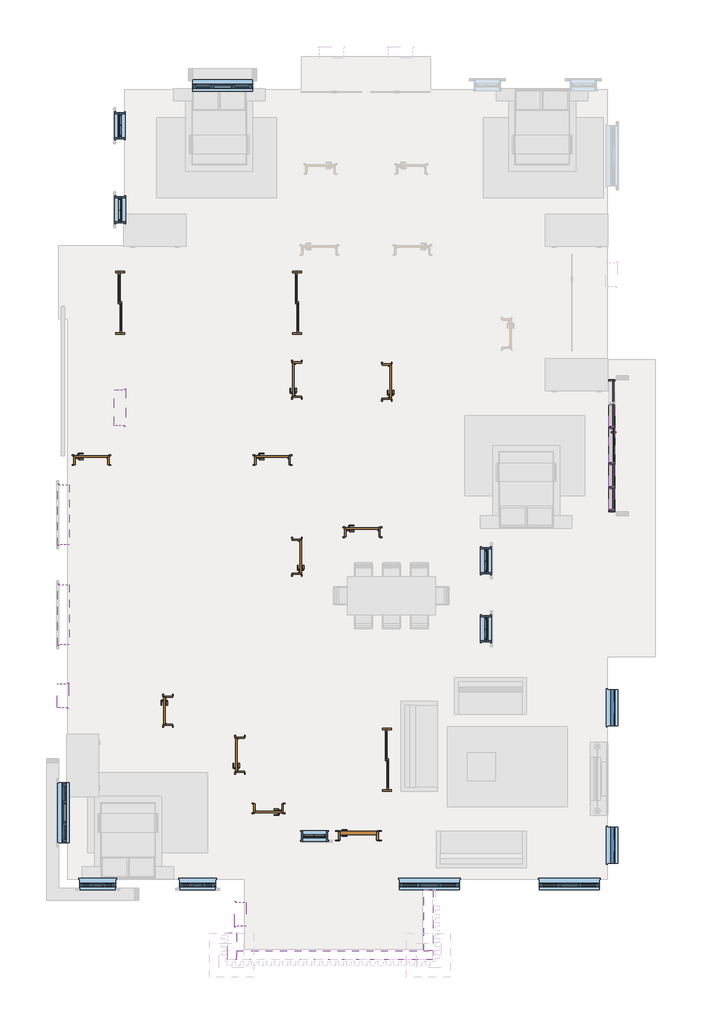
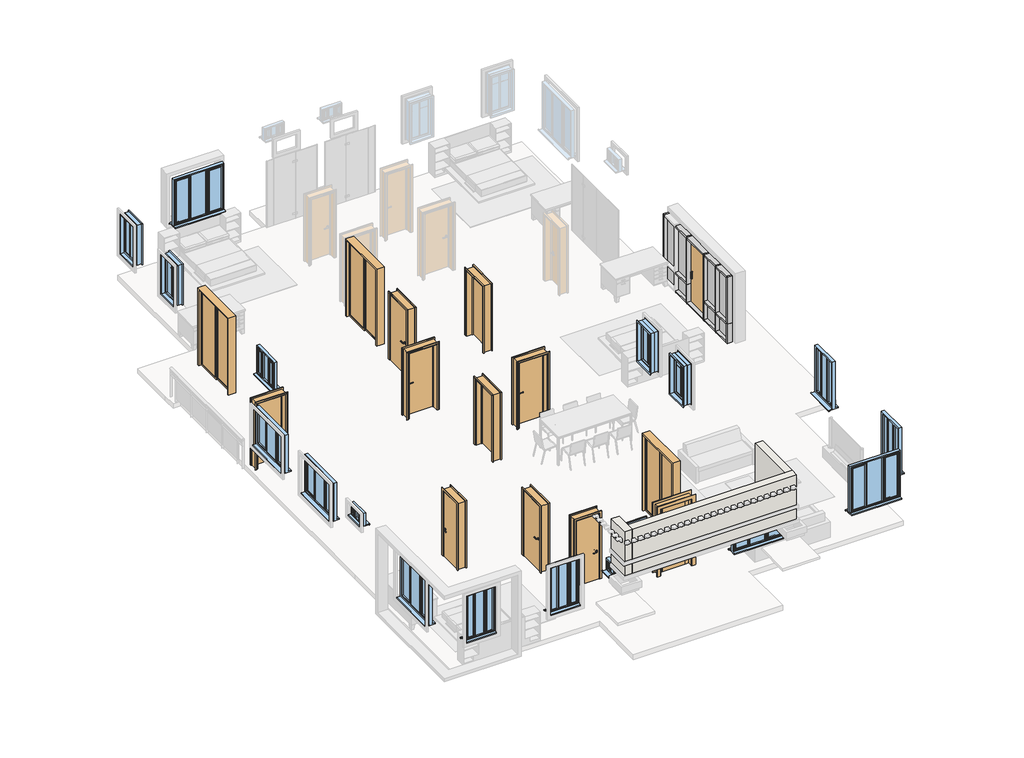
# One storey, part 1 of 2: 20 members, 18 windows, 14 doors, 8 plates, 3 walls.
"""IFC4 building model written with IfcOpenShell, lengths in millimetres."""

from ifc_helpers import new_model, si_unit, frame, origin, place, context, project, spatial, polyline, outline, extrude, faceted_brep, transform, mapped, element, save
from components import door_1500_x_2400mm_f3db478b, doors_intsgl_927b0b89, doors_intsgl_1caea894, doors_intsgl_900mm_doors_1c9cf9a6, doors_intsgl_900mm_doors_d21b38ee, m_door_curtain_wall_single_glass_m_door_curtain_wall_single_f8ee2cb8, single_flush_door_modern_12229_930_x_2100mm_fac4ccff, rectangular_mullion_50_x_150mm_5b5377e9, rectangular_mullion_50_x_150mm_de2b7ee4, rectangular_mullion_50_x_150mm_8a69f4a4, rectangular_mullion_50_x_150mm_b8dbbb25, rectangular_mullion_50_x_150mm_5dbd0429, rectangular_mullion_50_x_150mm_324a6438, rectangular_mullion_50_x_150mm_63369cdd, rectangular_mullion_50_x_150mm_7b69be1d, rectangular_mullion_50_x_150mm_c6835c94, system_panel_glazed_d134efab, system_panel_glazed_ea2acdbe, system_panel_glazed_163e0323, system_panel_glazed_68fefaed, tpl_plain_1500mm_wind_d4a9cd4c, tpl_plain_1500mm_wind_2_30e43110, tpl_plain_600mm_window_e9a44080, tpl_plain_900mm_wind_8db11632, tpl_plain_900mm_wind_2_fce8a64c, yu_window_casement_600x1200_84df8a12

model = new_model("IFC4")

# Units and contexts
model_context = context("Model", 3, world=origin())
ifc_project = project(units=[si_unit("LENGTHUNIT", "METRE", prefix="MILLI")], contexts=[model_context])

# Site, building, storey
site = spatial("IfcSite", under=ifc_project)
building = spatial("IfcBuilding", under=site)
storey = spatial("IfcBuildingStorey", under=building, Elevation=450.0)

# Doors
placement = place(None, origin())
door_1500_x_2400mm_shape = door_1500_x_2400mm_f3db478b(model_context)
element("IfcDoor", 1, ObjectType="1500 x 2400mm", at=placement, inside=storey, context=model_context, shape_type="MappedRepresentation", body=[
    mapped(door_1500_x_2400mm_shape, transform((-149.2953966, 3626.5650849, 450.0), x_axis=(0.0, -1.0, 0.0), y_axis=(1.0, 0.0, 0.0), z_axis=(0.0, 0.0, 1.0))),
])
element("IfcDoor", 2, ObjectType="1500 x 2400mm", at=placement, inside=storey, context=model_context, shape_type="MappedRepresentation", body=[
    mapped(door_1500_x_2400mm_shape, transform((-4574.2953966, 3626.5650849, 450.0), x_axis=(0.0, -1.0, 0.0), y_axis=(1.0, 0.0, 0.0), z_axis=(0.0, 0.0, 1.0))),
])
element("IfcDoor", 3, ObjectType="1500 x 2400mm", at=placement, inside=storey, context=model_context, shape_type="MappedRepresentation", body=[
    mapped(door_1500_x_2400mm_shape, transform((2100.7046034, -7795.9349151, 450.0), x_axis=(0.0, -1.0, 0.0), y_axis=(1.0, 0.0, 0.0), z_axis=(0.0, 0.0, 1.0))),
])
doors_intsgl_shape = doors_intsgl_927b0b89(model_context)
element("IfcDoor", 4, ObjectType="Doors_IntSgl", at=placement, inside=storey, context=model_context, shape_type="MappedRepresentation", body=[
    mapped(doors_intsgl_shape, transform((-3374.2953966, -6659.1929163, 450.0), x_axis=(0.0, -1.0, 0.0), y_axis=(1.0, 0.0, 0.0), z_axis=(0.0, 0.0, 1.0))),
])
doors_intsgl_2_shape = doors_intsgl_1caea894(model_context)
element("IfcDoor", 5, ObjectType="Doors_IntSgl", at=placement, inside=storey, context=model_context, shape_type="MappedRepresentation", body=[
    mapped(doors_intsgl_2_shape, transform((-861.7953966, -9096.6929163, 450.0), x_axis=(-1.0, 0.0, 0.0), y_axis=(0.0, -1.0, 0.0), z_axis=(0.0, 0.0, 1.0))),
])
doors_intsgl_900mm_doors_shape = doors_intsgl_900mm_doors_1c9cf9a6(model_context)
element("IfcDoor", 6, ObjectType="Doors_IntSgl : 900mm DOORS", at=placement, inside=storey, context=model_context, shape_type="MappedRepresentation", body=[
    mapped(doors_intsgl_900mm_doors_shape, transform((-5286.7953966, -396.6929163, 450.0), x_axis=(1.0, 0.0, 0.0), y_axis=(0.0, 1.0, 0.0), z_axis=(0.0, 0.0, 1.0))),
])
element("IfcDoor", 7, ObjectType="Doors_IntSgl : 900mm DOORS", at=placement, inside=storey, context=model_context, shape_type="MappedRepresentation", body=[
    mapped(doors_intsgl_900mm_doors_shape, transform((-761.7953966, -396.6929163, 450.0), x_axis=(1.0, 0.0, 0.0), y_axis=(0.0, 1.0, 0.0), z_axis=(0.0, 0.0, 1.0))),
])
element("IfcDoor", 8, ObjectType="Doors_IntSgl : 900mm DOORS", at=placement, inside=storey, context=model_context, shape_type="MappedRepresentation", body=[
    mapped(doors_intsgl_900mm_doors_shape, transform((1488.2046034, -2196.6929163, 450.0), x_axis=(1.0, 0.0, 0.0), y_axis=(0.0, 1.0, 0.0), z_axis=(0.0, 0.0, 1.0))),
])
element("IfcDoor", 9, ObjectType="Doors_IntSgl : 900mm DOORS", at=placement, inside=storey, context=model_context, shape_type="MappedRepresentation", body=[
    mapped(doors_intsgl_900mm_doors_shape, transform((-1574.2953966, -7759.1929163, 450.0), x_axis=(0.0, 1.0, 0.0), y_axis=(-1.0, 0.0, 0.0), z_axis=(0.0, 0.0, 1.0))),
])
element("IfcDoor", 10, ObjectType="Doors_IntSgl : 900mm DOORS", at=placement, inside=storey, context=model_context, shape_type="MappedRepresentation", body=[
    mapped(doors_intsgl_900mm_doors_shape, transform((-149.2953966, 1615.8070837, 450.0), x_axis=(0.0, 1.0, 0.0), y_axis=(-1.0, 0.0, 0.0), z_axis=(0.0, 0.0, 1.0))),
])
doors_intsgl_900mm_doors_2_shape = doors_intsgl_900mm_doors_d21b38ee(model_context)
element("IfcDoor", 11, ObjectType="Doors_IntSgl : 900mm DOORS", at=placement, inside=storey, context=model_context, shape_type="MappedRepresentation", body=[
    mapped(doors_intsgl_900mm_doors_2_shape, transform((-149.2953966, -2809.1929163, 450.0), x_axis=(0.0, 1.0, 0.0), y_axis=(-1.0, 0.0, 0.0), z_axis=(0.0, 0.0, 1.0))),
])
element("IfcDoor", 12, ObjectType="Doors_IntSgl : 900mm DOORS", at=placement, inside=storey, context=model_context, shape_type="MappedRepresentation", body=[
    mapped(doors_intsgl_900mm_doors_2_shape, transform((2100.7046034, 1565.8070837, 450.0), x_axis=(0.0, 1.0, 0.0), y_axis=(-1.0, 0.0, 0.0), z_axis=(0.0, 0.0, 1.0))),
])
m_door_curtain_wall_single_glass_m_door_curtain_wall_single_shape = m_door_curtain_wall_single_glass_m_door_curtain_wall_single_f8ee2cb8(model_context)
element("IfcDoor", 13, ObjectType="M_Door-Curtain-Wall-Single-Glass : M_Door-Curtain-Wall-Single-Glass", at=placement, inside=storey, context=model_context, shape_type="MappedRepresentation", body=[
    mapped(m_door_curtain_wall_single_glass_m_door_curtain_wall_single_shape, transform((7725.7046034, -34.1929163, 500.0), x_axis=(0.0, -1.0, 0.0), y_axis=(1.0, 0.0, 0.0), z_axis=(0.0, 0.0, 1.0))),
])
single_flush_door_modern_12229_930_x_2100mm_shape = single_flush_door_modern_12229_930_x_2100mm_fac4ccff(model_context)
element("IfcDoor", 14, ObjectType="Single_Flush_Door_-_Modern_12229 : 930 x 2100mm", at=placement, inside=storey, context=model_context, shape_type="MappedRepresentation", body=[
    mapped(single_flush_door_modern_12229_930_x_2100mm_shape, transform((1388.2046034, -9784.1929163, 450.0), x_axis=(-1.0, 0.0, 0.0), y_axis=(0.0, -1.0, 0.0), z_axis=(0.0, 0.0, 1.0))),
])

# Members
rectangular_mullion_50_x_150mm_shape = rectangular_mullion_50_x_150mm_5b5377e9(model_context)
element("IfcMember", 15, ObjectType="Rectangular Mullion : 50 x 150mm", at=placement, inside=storey, context=model_context, shape_type="MappedRepresentation", body=[
    mapped(rectangular_mullion_50_x_150mm_shape, transform((7725.7046034, -1634.1929163, 2550.0), x_axis=(0.0, 0.0, 1.0), y_axis=(-1.0, 0.0, 0.0), z_axis=(0.0, -1.0, 0.0))),
])
element("IfcMember", 16, ObjectType="Rectangular Mullion : 50 x 150mm", at=placement, inside=storey, context=model_context, shape_type="MappedRepresentation", body=[
    mapped(rectangular_mullion_50_x_150mm_shape, transform((7725.7046034, -1109.1929163, 450.0), x_axis=(0.0, 0.0, -1.0), y_axis=(-1.0, 0.0, 0.0), z_axis=(0.0, 1.0, 0.0))),
])
rectangular_mullion_50_x_150mm_2_shape = rectangular_mullion_50_x_150mm_de2b7ee4(model_context)
element("IfcMember", 17, ObjectType="Rectangular Mullion : 50 x 150mm", at=placement, inside=storey, context=model_context, shape_type="MappedRepresentation", body=[
    mapped(rectangular_mullion_50_x_150mm_2_shape, transform((7725.7046034, -1084.1929163, 450.0), x_axis=(0.0, -1.0, 0.0), y_axis=(-1.0, 0.0, 0.0), z_axis=(0.0, 0.0, -1.0))),
])
element("IfcMember", 18, ObjectType="Rectangular Mullion : 50 x 150mm", at=placement, inside=storey, context=model_context, shape_type="MappedRepresentation", body=[
    mapped(rectangular_mullion_50_x_150mm_2_shape, transform((7725.7046034, -484.1929163, 450.0), x_axis=(0.0, -1.0, 0.0), y_axis=(-1.0, 0.0, 0.0), z_axis=(0.0, 0.0, -1.0))),
])
element("IfcMember", 19, ObjectType="Rectangular Mullion : 50 x 150mm", at=placement, inside=storey, context=model_context, shape_type="MappedRepresentation", body=[
    mapped(rectangular_mullion_50_x_150mm_2_shape, transform((7725.7046034, 415.8070837, 450.0), x_axis=(0.0, -1.0, 0.0), y_axis=(-1.0, 0.0, 0.0), z_axis=(0.0, 0.0, -1.0))),
])
rectangular_mullion_50_x_150mm_3_shape = rectangular_mullion_50_x_150mm_8a69f4a4(model_context)
element("IfcMember", 20, ObjectType="Rectangular Mullion : 50 x 150mm", at=placement, inside=storey, context=model_context, shape_type="MappedRepresentation", body=[
    mapped(rectangular_mullion_50_x_150mm_3_shape, transform((7725.7046034, -1634.1929163, 1060.0), x_axis=(0.0, 0.0, 1.0), y_axis=(-1.0, 0.0, 0.0), z_axis=(0.0, -1.0, 0.0))),
])
rectangular_mullion_50_x_150mm_4_shape = rectangular_mullion_50_x_150mm_b8dbbb25(model_context)
element("IfcMember", 21, ObjectType="Rectangular Mullion : 50 x 150mm", at=placement, inside=storey, context=model_context, shape_type="MappedRepresentation", body=[
    mapped(rectangular_mullion_50_x_150mm_4_shape, transform((7725.7046034, -1059.1929163, 1060.0), x_axis=(0.0, 0.0, 1.0), y_axis=(-1.0, 0.0, 0.0), z_axis=(0.0, -1.0, 0.0))),
])
element("IfcMember", 22, ObjectType="Rectangular Mullion : 50 x 150mm", at=placement, inside=storey, context=model_context, shape_type="MappedRepresentation", body=[
    mapped(rectangular_mullion_50_x_150mm_4_shape, transform((7725.7046034, 440.8070837, 1060.0), x_axis=(0.0, 0.0, 1.0), y_axis=(-1.0, 0.0, 0.0), z_axis=(0.0, -1.0, 0.0))),
])
rectangular_mullion_50_x_150mm_5_shape = rectangular_mullion_50_x_150mm_5dbd0429(model_context)
element("IfcMember", 23, ObjectType="Rectangular Mullion : 50 x 150mm", at=placement, inside=storey, context=model_context, shape_type="MappedRepresentation", body=[
    mapped(rectangular_mullion_50_x_150mm_5_shape, transform((7725.7046034, -509.1929163, 450.0), x_axis=(0.0, 0.0, -1.0), y_axis=(-1.0, 0.0, 0.0), z_axis=(0.0, 1.0, 0.0))),
])
element("IfcMember", 24, ObjectType="Rectangular Mullion : 50 x 150mm", at=placement, inside=storey, context=model_context, shape_type="MappedRepresentation", body=[
    mapped(rectangular_mullion_50_x_150mm_5_shape, transform((7725.7046034, 990.8070837, 450.0), x_axis=(0.0, 0.0, -1.0), y_axis=(-1.0, 0.0, 0.0), z_axis=(0.0, 1.0, 0.0))),
])
rectangular_mullion_50_x_150mm_6_shape = rectangular_mullion_50_x_150mm_324a6438(model_context)
element("IfcMember", 25, ObjectType="Rectangular Mullion : 50 x 150mm", at=placement, inside=storey, context=model_context, shape_type="MappedRepresentation", body=[
    mapped(rectangular_mullion_50_x_150mm_6_shape, transform((7725.7046034, 390.8070837, 450.0), x_axis=(0.0, 0.0, -1.0), y_axis=(-1.0, 0.0, 0.0), z_axis=(0.0, 1.0, 0.0))),
])
element("IfcMember", 26, ObjectType="Rectangular Mullion : 50 x 150mm", at=placement, inside=storey, context=model_context, shape_type="MappedRepresentation", body=[
    mapped(rectangular_mullion_50_x_150mm_5_shape, transform((7725.7046034, -1059.1929163, 2550.0), x_axis=(0.0, 0.0, 1.0), y_axis=(-1.0, 0.0, 0.0), z_axis=(0.0, -1.0, 0.0))),
])
element("IfcMember", 27, ObjectType="Rectangular Mullion : 50 x 150mm", at=placement, inside=storey, context=model_context, shape_type="MappedRepresentation", body=[
    mapped(rectangular_mullion_50_x_150mm_5_shape, transform((7725.7046034, 440.8070837, 2550.0), x_axis=(0.0, 0.0, 1.0), y_axis=(-1.0, 0.0, 0.0), z_axis=(0.0, -1.0, 0.0))),
])
element("IfcMember", 28, ObjectType="Rectangular Mullion : 50 x 150mm", at=placement, inside=storey, context=model_context, shape_type="MappedRepresentation", body=[
    mapped(rectangular_mullion_50_x_150mm_6_shape, transform((7725.7046034, -459.1929163, 2550.0), x_axis=(0.0, 0.0, 1.0), y_axis=(-1.0, 0.0, 0.0), z_axis=(0.0, -1.0, 0.0))),
])
rectangular_mullion_50_x_150mm_7_shape = rectangular_mullion_50_x_150mm_63369cdd(model_context)
element("IfcMember", 29, ObjectType="Rectangular Mullion : 50 x 150mm", at=placement, inside=storey, context=model_context, shape_type="MappedRepresentation", body=[
    mapped(rectangular_mullion_50_x_150mm_7_shape, transform((7725.7046034, -1084.1929163, 1060.0), x_axis=(0.0, -1.0, 0.0), y_axis=(-1.0, 0.0, 0.0), z_axis=(0.0, 0.0, -1.0))),
])
element("IfcMember", 30, ObjectType="Rectangular Mullion : 50 x 150mm", at=placement, inside=storey, context=model_context, shape_type="MappedRepresentation", body=[
    mapped(rectangular_mullion_50_x_150mm_7_shape, transform((7725.7046034, -484.1929163, 1060.0), x_axis=(0.0, -1.0, 0.0), y_axis=(-1.0, 0.0, 0.0), z_axis=(0.0, 0.0, -1.0))),
])
element("IfcMember", 31, ObjectType="Rectangular Mullion : 50 x 150mm", at=placement, inside=storey, context=model_context, shape_type="MappedRepresentation", body=[
    mapped(rectangular_mullion_50_x_150mm_7_shape, transform((7725.7046034, 415.8070837, 1060.0), x_axis=(0.0, -1.0, 0.0), y_axis=(-1.0, 0.0, 0.0), z_axis=(0.0, 0.0, -1.0))),
])
rectangular_mullion_50_x_150mm_8_shape = rectangular_mullion_50_x_150mm_7b69be1d(model_context)
element("IfcMember", 32, ObjectType="Rectangular Mullion : 50 x 150mm", at=placement, inside=storey, context=model_context, shape_type="MappedRepresentation", body=[
    mapped(rectangular_mullion_50_x_150mm_8_shape, transform((7725.7046034, 1615.8070837, 2550.0), x_axis=(0.0, 1.0, 0.0), y_axis=(-1.0, 0.0, 0.0), z_axis=(0.0, 0.0, 1.0))),
])
rectangular_mullion_50_x_150mm_9_shape = rectangular_mullion_50_x_150mm_c6835c94(model_context)
element("IfcMember", 33, ObjectType="Rectangular Mullion : 50 x 150mm", at=placement, inside=storey, context=model_context, shape_type="MappedRepresentation", body=[
    mapped(rectangular_mullion_50_x_150mm_9_shape, transform((7725.7046034, -1684.1929163, 450.0), x_axis=(0.0, -1.0, 0.0), y_axis=(-1.0, 0.0, 0.0), z_axis=(0.0, 0.0, -1.0))),
])
element("IfcMember", 34, ObjectType="Rectangular Mullion : 50 x 150mm", at=placement, inside=storey, context=model_context, shape_type="MappedRepresentation", body=[
    mapped(rectangular_mullion_50_x_150mm_8_shape, transform((7725.7046034, -1684.1929163, 1060.0), x_axis=(0.0, -1.0, 0.0), y_axis=(-1.0, 0.0, 0.0), z_axis=(0.0, 0.0, -1.0))),
])

# Plates
system_panel_glazed_shape = system_panel_glazed_d134efab(model_context)
element("IfcPlate", 35, ObjectType="System Panel : Glazed", at=placement, inside=storey, context=model_context, shape_type="MappedRepresentation", body=[
    mapped(system_panel_glazed_shape, transform((7725.7046034, 1303.3070837, 500.0), x_axis=(0.0, -1.0, 0.0), y_axis=(1.0, 0.0, 0.0), z_axis=(0.0, 0.0, 1.0))),
])
element("IfcPlate", 36, ObjectType="System Panel : Glazed", at=placement, inside=storey, context=model_context, shape_type="MappedRepresentation", body=[
    mapped(system_panel_glazed_shape, transform((7725.7046034, -1371.6929163, 500.0), x_axis=(0.0, -1.0, 0.0), y_axis=(1.0, 0.0, 0.0), z_axis=(0.0, 0.0, 1.0))),
])
system_panel_glazed_2_shape = system_panel_glazed_ea2acdbe(model_context)
element("IfcPlate", 37, ObjectType="System Panel : Glazed", at=placement, inside=storey, context=model_context, shape_type="MappedRepresentation", body=[
    mapped(system_panel_glazed_2_shape, transform((7725.7046034, -784.1929163, 500.0), x_axis=(0.0, -1.0, 0.0), y_axis=(1.0, 0.0, 0.0), z_axis=(0.0, 0.0, 1.0))),
])
element("IfcPlate", 38, ObjectType="System Panel : Glazed", at=placement, inside=storey, context=model_context, shape_type="MappedRepresentation", body=[
    mapped(system_panel_glazed_2_shape, transform((7725.7046034, 715.8070837, 500.0), x_axis=(0.0, -1.0, 0.0), y_axis=(1.0, 0.0, 0.0), z_axis=(0.0, 0.0, 1.0))),
])
system_panel_glazed_3_shape = system_panel_glazed_163e0323(model_context)
element("IfcPlate", 39, ObjectType="System Panel : Glazed", at=placement, inside=storey, context=model_context, shape_type="MappedRepresentation", body=[
    mapped(system_panel_glazed_3_shape, transform((7725.7046034, 1303.3070837, 1085.0), x_axis=(0.0, -1.0, 0.0), y_axis=(1.0, 0.0, 0.0), z_axis=(0.0, 0.0, 1.0))),
])
element("IfcPlate", 40, ObjectType="System Panel : Glazed", at=placement, inside=storey, context=model_context, shape_type="MappedRepresentation", body=[
    mapped(system_panel_glazed_3_shape, transform((7725.7046034, -1371.6929163, 1085.0), x_axis=(0.0, -1.0, 0.0), y_axis=(1.0, 0.0, 0.0), z_axis=(0.0, 0.0, 1.0))),
])
system_panel_glazed_4_shape = system_panel_glazed_68fefaed(model_context)
element("IfcPlate", 41, ObjectType="System Panel : Glazed", at=placement, inside=storey, context=model_context, shape_type="MappedRepresentation", body=[
    mapped(system_panel_glazed_4_shape, transform((7725.7046034, 715.8070837, 1085.0), x_axis=(0.0, -1.0, 0.0), y_axis=(1.0, 0.0, 0.0), z_axis=(0.0, 0.0, 1.0))),
])
element("IfcPlate", 42, ObjectType="System Panel : Glazed", at=placement, inside=storey, context=model_context, shape_type="MappedRepresentation", body=[
    mapped(system_panel_glazed_4_shape, transform((7725.7046034, -784.1929163, 1085.0), x_axis=(0.0, -1.0, 0.0), y_axis=(1.0, 0.0, 0.0), z_axis=(0.0, 0.0, 1.0))),
])

# Walls
element("IfcWall", 43, ObjectType="225 wall", at=placement, inside=storey, context=model_context, shape_type="Brep", body=[
    faceted_brep([(-1879.2953966, -12209.1929163, 3150.0), (-1879.2953966, -12886.6929163, 3150.0), (-1879.2953966, -12886.6929163, 4650.0), (-1879.2953966, -12209.1929163, 4650.0), (-1654.2953966, -12209.1929163, 3150.0), (-1654.2953966, -12209.1929163, 4650.0), (-1654.2953966, -12661.6929163, 4650.0), (-1654.2953966, -12886.6929163, 4650.0), (-1654.2953966, -12886.6929163, 3150.0), (-1654.2953966, -12661.6929163, 3150.0)], [[[0, 1, 2, 3]], [[4, 5, 6, 7, 8, 9]], [[1, 0, 4, 9, 8]], [[3, 2, 7, 6, 5]], [[0, 3, 5, 4]], [[2, 1, 8, 7]]]),
])
element("IfcWall", 44, ObjectType="225 wall", at=placement, inside=storey, context=model_context, shape_type="Brep", body=[
    faceted_brep([(-1654.2953966, -12886.6929163, 3150.0), (3255.7046034, -12886.6929163, 3150.0), (3255.7046034, -12886.6929163, 4650.0), (-1654.2953966, -12886.6929163, 4650.0), (-1654.2953966, -12661.6929163, 3150.0), (-1654.2953966, -12661.6929163, 4650.0), (3030.7046034, -12661.6929163, 4650.0), (3255.7046034, -12661.6929163, 4650.0), (3255.7046034, -12661.6929163, 3150.0), (3030.7046034, -12661.6929163, 3150.0)], [[[0, 1, 2, 3]], [[4, 5, 6, 7, 8, 9]], [[1, 0, 4, 9, 8]], [[3, 2, 7, 6, 5]], [[0, 3, 5, 4]], [[2, 1, 8, 7]]]),
])
element("IfcWall", 45, ObjectType="225 wall", at=placement, inside=storey, context=model_context, shape_type="SweptSolid", body=[
    extrude(outline(polyline([(3030.7046034, -12661.6929163), (3030.7046034, -11134.1929163), (3255.7046034, -11134.1929163), (3255.7046034, -12661.6929163), (3030.7046034, -12661.6929163)])), frame((0.0, 0.0, 3150.0), z_axis=(0.0, 0.0, 1.0), x_axis=(1.0, 0.0, 0.0)), (0.0, 0.0, 1.0), 1500.0),
])

# Windows
tpl_plain_1500mm_wind_shape = tpl_plain_1500mm_wind_d4a9cd4c(model_context)
element("IfcWindow", 46, ObjectType="Tpl Plain : 1500mm wind", at=placement, inside=storey, context=model_context, shape_type="MappedRepresentation", body=[
    mapped(tpl_plain_1500mm_wind_shape, transform((-2536.7953966, 8986.7636515, 450.0), x_axis=(-1.0, 0.0, 0.0), y_axis=(0.0, -1.0, 0.0), z_axis=(0.0, 0.0, 1.0))),
])
element("IfcWindow", 47, ObjectType="Tpl Plain : 1500mm wind", at=placement, inside=storey, context=model_context, shape_type="MappedRepresentation", body=[
    mapped(tpl_plain_1500mm_wind_shape, transform((-6007.7519645, -9734.1929163, 450.0), x_axis=(0.0, -1.0, 0.0), y_axis=(1.0, 0.0, 0.0), z_axis=(0.0, 0.0, 1.0))),
])
element("IfcWindow", 48, ObjectType="Tpl Plain : 1500mm wind", at=placement, inside=storey, context=model_context, shape_type="MappedRepresentation", body=[
    mapped(tpl_plain_1500mm_wind_shape, transform((2638.2046034, -10975.7363485, 450.0), x_axis=(-1.0, 0.0, 0.0), y_axis=(0.0, -1.0, 0.0), z_axis=(0.0, 0.0, 1.0))),
])
element("IfcWindow", 49, ObjectType="Tpl Plain : 1500mm wind", at=placement, inside=storey, context=model_context, shape_type="MappedRepresentation", body=[
    mapped(tpl_plain_1500mm_wind_shape, transform((6138.2046034, -10975.7363485, 450.0), x_axis=(-1.0, 0.0, 0.0), y_axis=(0.0, -1.0, 0.0), z_axis=(0.0, 0.0, 1.0))),
])
tpl_plain_1500mm_wind_2_shape = tpl_plain_1500mm_wind_2_30e43110(model_context)
element("IfcWindow", 50, ObjectType="Tpl Plain : 1500mm wind 2", at=placement, inside=storey, context=model_context, shape_type="MappedRepresentation", body=[
    mapped(tpl_plain_1500mm_wind_2_shape, transform((-6007.7519645, -2284.1929163, 450.0), x_axis=(0.0, -1.0, 0.0), y_axis=(1.0, 0.0, 0.0), z_axis=(0.0, 0.0, 1.0))),
])
element("IfcWindow", 51, ObjectType="Tpl Plain : 1500mm wind 2", at=placement, inside=storey, context=model_context, shape_type="MappedRepresentation", body=[
    mapped(tpl_plain_1500mm_wind_2_shape, transform((-6007.7519645, -4784.1929163, 450.0), x_axis=(0.0, -1.0, 0.0), y_axis=(1.0, 0.0, 0.0), z_axis=(0.0, 0.0, 1.0))),
])
tpl_plain_600mm_window_shape = tpl_plain_600mm_window_e9a44080(model_context)
element("IfcWindow", 52, ObjectType="Tpl Plain : 600mm window", at=placement, inside=storey, context=model_context, shape_type="MappedRepresentation", body=[
    mapped(tpl_plain_600mm_window_shape, transform((-1582.7519645, -12119.1929163, 450.0), x_axis=(0.0, -1.0, 0.0), y_axis=(1.0, 0.0, 0.0), z_axis=(0.0, 0.0, 1.0))),
])
element("IfcWindow", 53, ObjectType="Tpl Plain : 600mm window", at=placement, inside=storey, context=model_context, shape_type="MappedRepresentation", body=[
    mapped(tpl_plain_600mm_window_shape, transform((-5990.8388288, -5909.1929163, 450.0), x_axis=(0.0, 1.0, 0.0), y_axis=(-1.0, 0.0, 0.0), z_axis=(0.0, 0.0, 1.0))),
])
tpl_plain_900mm_wind_shape = tpl_plain_900mm_wind_8db11632(model_context)
element("IfcWindow", 54, ObjectType="Tpl Plain : 900mm wind", at=placement, inside=storey, context=model_context, shape_type="MappedRepresentation", body=[
    mapped(tpl_plain_900mm_wind_shape, transform((-4565.8388288, 1340.8070837, 450.0), x_axis=(0.0, 1.0, 0.0), y_axis=(-1.0, 0.0, 0.0), z_axis=(0.0, 0.0, 1.0))),
])
tpl_plain_900mm_wind_2_shape = tpl_plain_900mm_wind_2_fce8a64c(model_context)
element("IfcWindow", 55, ObjectType="Tpl Plain : 900mm wind 2", at=placement, inside=storey, context=model_context, shape_type="MappedRepresentation", body=[
    mapped(tpl_plain_900mm_wind_2_shape, transform((7717.2480355, -10446.6929163, 690.0), x_axis=(0.0, -1.0, 0.0), y_axis=(1.0, 0.0, 0.0), z_axis=(0.0, 0.0, 1.0))),
])
element("IfcWindow", 56, ObjectType="Tpl Plain : 900mm wind 2", at=placement, inside=storey, context=model_context, shape_type="MappedRepresentation", body=[
    mapped(tpl_plain_900mm_wind_2_shape, transform((7717.2480355, -7009.1929163, 690.0), x_axis=(0.0, -1.0, 0.0), y_axis=(1.0, 0.0, 0.0), z_axis=(0.0, 0.0, 1.0))),
])
element("IfcWindow", 57, ObjectType="Tpl Plain : 900mm wind 2", at=placement, inside=storey, context=model_context, shape_type="MappedRepresentation", body=[
    mapped(tpl_plain_900mm_wind_2_shape, transform((-3061.7953966, -10975.7363485, 450.0), x_axis=(-1.0, 0.0, 0.0), y_axis=(0.0, -1.0, 0.0), z_axis=(0.0, 0.0, 1.0))),
])
element("IfcWindow", 58, ObjectType="Tpl Plain : 900mm wind 2", at=placement, inside=storey, context=model_context, shape_type="MappedRepresentation", body=[
    mapped(tpl_plain_900mm_wind_2_shape, transform((-5561.7953966, -10975.7363485, 450.0), x_axis=(-1.0, 0.0, 0.0), y_axis=(0.0, -1.0, 0.0), z_axis=(0.0, 0.0, 1.0))),
])
yu_window_casement_600x1200_shape = yu_window_casement_600x1200_84df8a12(model_context)
element("IfcWindow", 59, ObjectType="Yu_Window : Casement 600x1200", at=placement, inside=storey, context=model_context, shape_type="MappedRepresentation", body=[
    mapped(yu_window_casement_600x1200_shape, transform((-4574.2953966, 7965.8070837, 990.0), x_axis=(0.0, 1.0, 0.0), y_axis=(-1.0, 0.0, 0.0), z_axis=(0.0, 0.0, 1.0))),
])
element("IfcWindow", 60, ObjectType="Yu_Window : Casement 600x1200", at=placement, inside=storey, context=model_context, shape_type="MappedRepresentation", body=[
    mapped(yu_window_casement_600x1200_shape, transform((-4574.2953966, 5865.8070837, 990.0), x_axis=(0.0, -1.0, 0.0), y_axis=(1.0, 0.0, 0.0), z_axis=(0.0, 0.0, 1.0))),
])
element("IfcWindow", 61, ObjectType="Yu_Window : Casement 600x1200", at=placement, inside=storey, context=model_context, shape_type="MappedRepresentation", body=[
    mapped(yu_window_casement_600x1200_shape, transform((4575.7046034, -2909.1929163, 990.0), x_axis=(0.0, -1.0, 0.0), y_axis=(1.0, 0.0, 0.0), z_axis=(0.0, 0.0, 1.0))),
])
element("IfcWindow", 62, ObjectType="Yu_Window : Casement 600x1200", at=placement, inside=storey, context=model_context, shape_type="MappedRepresentation", body=[
    mapped(yu_window_casement_600x1200_shape, transform((4575.7046034, -4609.1929163, 990.0), x_axis=(0.0, -1.0, 0.0), y_axis=(1.0, 0.0, 0.0), z_axis=(0.0, 0.0, 1.0))),
])
element("IfcWindow", 63, ObjectType="Yu_Window : Casement 600x1200", at=placement, inside=storey, context=model_context, shape_type="MappedRepresentation", body=[
    mapped(yu_window_casement_600x1200_shape, transform((288.2046034, -9784.1929163, 450.0), x_axis=(-1.0, 0.0, 0.0), y_axis=(0.0, -1.0, 0.0), z_axis=(0.0, 0.0, 1.0))),
])

save(model, "model.ifc")

# Revit data of these elements
# Type "1500 x 2400mm"
#   Type Mark = "47"
#   Operation = "UserDefined"
#   Analytic Construction = "<None>"
#   Width = 1500 mm
#   Thickness = 40 mm
#   Rough Width = 1580 mm
#   Rough Height = 2440 mm
#   Panel Width = 777.5 mm
#   Panel Frame = 55 mm
#   Height = 2400 mm
#   Frame Depth = 40 mm
#   Define Thermal Properties by = 1
#   Glass Material = Sliding Door Glass
#   Frame Material = Sliding Door Frame
#   Function = (empty or 0)
# Type "Doors_IntSgl"
#   Type Mark = "45"
#   Type Comments = "Internal Single"
#   Operation = "SingleSwingRight"
#   Manufacturer = "Revit"
#   Keynote = "L20"
#   Description = "Internal Single Door"
#   Analytic Construction = "Metal"
#   UnderCut = 8 mm
#   Tolerance = 2 mm
#   Thickness = 38 mm
#   Thermal Resistance (R) = 0.270117 (m²·K)/W
#   Structural Tolerance = 8 mm
#   StopDepth = 32 mm
#   Stop Thickness = 19 mm
#   Rough Width = 750 mm
#   Rough Height = 2100 mm
#   Height to Top Lock Rail = 1000 mm
#   Heat Transfer Coefficient (U) = 3.7021 W/(m²·K)
#   Handle Z Distance = 900 mm
#   Handle X Distance = 75 mm
#   Frame Thickness = 32 mm
#   Door Panel Width = 666 mm
#   Door Panel Thickness = 38 mm
#   Door Panel Offset = 0 mm
#   Height = 2100 mm
#   Width = 750 mm
#   Door Panel Height = 2050 mm
#   Architrave Setback = 5 mm
#   Vis - Ironmongery = yes
#   Define Thermal Properties by = 1
#   Material Ironmongery = Door - Handle
#   Material Frame = Door - Frame/Mullion (1)
#   Material Door = Door - Panel
#   Material Architrave = Door - Architrave
#   Visual Light Transmittance = 0
#   Solar Heat Gain Coefficient = 0
#   Function = (empty or 0)
#   Wall Closure = (empty or 0)
# Type "Doors_IntSgl : 900mm DOORS"
#   Type Mark = "46"
#   Type Comments = "Internal Single"
#   Operation = "SingleSwingRight"
#   Manufacturer = "Revit"
#   Keynote = "L20"
#   Description = "Internal Single Door"
#   Analytic Construction = "Metal"
#   UnderCut = 8 mm
#   Tolerance = 2 mm
#   Thickness = 38 mm
#   Thermal Resistance (R) = 0.270117 (m²·K)/W
#   Structural Tolerance = 8 mm
#   StopDepth = 32 mm
#   Stop Thickness = 19 mm
#   Rough Width = 900 mm
#   Rough Height = 2100 mm
#   Height to Top Lock Rail = 1000 mm
#   Heat Transfer Coefficient (U) = 3.7021 W/(m²·K)
#   Handle Z Distance = 1000 mm
#   Handle X Distance = 75 mm
#   Frame Thickness = 32 mm
#   Door Panel Width = 816 mm
#   Door Panel Thickness = 38 mm
#   Door Panel Offset = 0 mm
#   Height = 2100 mm
#   Width = 900 mm
#   Door Panel Height = 2050 mm
#   Architrave Setback = 5 mm
#   Vis - Ironmongery = yes
#   Define Thermal Properties by = 1
#   Material Ironmongery = Door - Handle
#   Material Frame = Door - Frame/Mullion (1)
#   Material Door = Door - Panel
#   Material Architrave = Door - Architrave
#   Visual Light Transmittance = 0
#   Solar Heat Gain Coefficient = 0
#   Function = (empty or 0)
#   Wall Closure = (empty or 0)
# Type "M_Door-Curtain-Wall-Single-Glass : M_Door-Curtain-Wall-Single-Glass"
#   Type Mark = "51"
#   Assembly Code = "B2030100"
#   Analytic Construction = "<None>"
#   Width [instance default] = 900 mm
#   Thermal Resistance (R) = 1.7611 (m²·K)/W
#   Swing Angle [instance default] = 90.00°
#   Heat Transfer Coefficient (U) = 0.567826 W/(m²·K)
#   Offset = 50.8 mm
#   Define Thermal Properties by = 1
#   Function = 1
#   Door Handle Material = Aluminum
#   Glazing = Glass
#   Visual Light Transmittance = 0
#   Solar Heat Gain Coefficient = 0
#   Construction Type Id = ""
# Type "Single_Flush_Door_-_Modern_12229 : 930 x 2100mm"
#   Type Mark = "50"
#   Description = "HWD FRAMED & PANELLED SINGLE DOOR"
#   Analytic Construction = "<None>"
#   Thickness = 45 mm
#   Rough Width = 1000 mm
#   Rough Height = 2145 mm
#   Frame Projection Ext. = 10 mm
#   Frame Projection Int. = 10 mm
#   Frame Width = 75 mm
#   Height = 2100 mm
#   Width = 930 mm
#   Define Thermal Properties by = 1
#   Jamb Material = Window Frame
#   Door Material = Window Frame
#   Function = (empty or 0)
#   Wall Closure = (empty or 0)
#   Assembly Code = ""
# Type "Rectangular Mullion : 50 x 150mm"
#   built-in parameter 1007304 = 0.492126 (stored number, unit not read)
#   built-in parameter 1007301 = 0.082021 (stored number, unit not read)
#   built-in parameter 1007300 = 0.082021 (stored number, unit not read)
# Type "System Panel : Glazed"
#   Construction Type Id = "GSP4R"
#   Analytic Construction = "1/8 in Pilkington single glazing"
#   Visual Light Transmittance = 0.9
#   Solar Heat Gain Coefficient = 0.86
#   Heat Transfer Coefficient (U) = 6.7069 W/(m²·K)
#   Define Thermal Properties by = 1
# Type "225 wall"
#   Layers, outside or top first: 225 mm "Concrete, Cast In Situ" (function 1)
# Type "Tpl Plain : 1500mm wind"
#   Type Mark = "34"
#   Operation = "TriplePanelVertical"
#   Manufacturer = "Revit"
#   Keynote = "L10"
#   Analytic Construction = "<None>"
#   Wrap Layers (Ext) from Ext = 102.5 mm
#   Wrap Layers (Int) from Ext = 177.5 mm
#   Window Board Projection = 25 mm
#   Window Board Extension = 25 mm
#   Rough Width = 1500 mm
#   Rough Height = 1500 mm
#   Height = 1500 mm
#   Width = 1500 mm
#   Glazing Thickness = 24 mm
#   FrameOffset - External = 50 mm
#   Frame Depth = 65 mm
#   Default Head Height = 2400 mm
#   Cill Depth = 87.5 mm
#   Cavity Closer Width = 50 mm
#   Cavity Closer Offset from Ext = 102.5 mm
#   Cavity Closer Depth = 85 mm
#   Vis - Cavity Closers = yes
#   Define Thermal Properties by = 1
#   Material Trim = Window Frame
#   Material Glass = Glass
#   Material Frame = Window Frame
#   Wall Closure = (empty or 0)
# Type "Tpl Plain : 1500mm wind 2"
#   Type Mark = "37"
#   Operation = "TriplePanelVertical"
#   Manufacturer = "Revit"
#   Keynote = "L10"
#   Analytic Construction = "<None>"
#   Wrap Layers (Ext) from Ext = 102.5 mm
#   Wrap Layers (Int) from Ext = 177.5 mm
#   Window Board Projection = 25 mm
#   Window Board Extension = 25 mm
#   Rough Width = 1500 mm
#   Rough Height = 1200 mm
#   Height = 1200 mm
#   Width = 1500 mm
#   Glazing Thickness = 24 mm
#   FrameOffset - External = 50 mm
#   Frame Depth = 65 mm
#   Default Head Height = 2400 mm
#   Cill Depth = 87.5 mm
#   Cavity Closer Width = 50 mm
#   Cavity Closer Offset from Ext = 102.5 mm
#   Cavity Closer Depth = 85 mm
#   Vis - Cavity Closers = yes
#   Define Thermal Properties by = 1
#   Material Trim = Window Frame
#   Material Glass = Glass
#   Material Frame = Window Frame
#   Wall Closure = (empty or 0)
# Type "Tpl Plain : 600mm window"
#   Type Mark = "33"
#   Operation = "TriplePanelVertical"
#   Manufacturer = "Revit"
#   Keynote = "L10"
#   Analytic Construction = "<None>"
#   Wrap Layers (Ext) from Ext = 102.5 mm
#   Wrap Layers (Int) from Ext = 177.5 mm
#   Window Board Projection = 25 mm
#   Window Board Extension = 25 mm
#   Rough Width = 600 mm
#   Rough Height = 400 mm
#   Height = 400 mm
#   Width = 600 mm
#   Glazing Thickness = 24 mm
#   FrameOffset - External = 50 mm
#   Frame Depth = 65 mm
#   Default Head Height = 2400 mm
#   Cill Depth = 87.5 mm
#   Cavity Closer Width = 50 mm
#   Cavity Closer Offset from Ext = 102.5 mm
#   Cavity Closer Depth = 85 mm
#   Vis - Cavity Closers = yes
#   Define Thermal Properties by = 1
#   Material Trim = Window Frame
#   Material Glass = Glass
#   Material Frame = Window Frame
#   Wall Closure = (empty or 0)
# Type "Tpl Plain : 900mm wind"
#   Type Mark = "35"
#   Operation = "TriplePanelVertical"
#   Manufacturer = "Revit"
#   Keynote = "L10"
#   Analytic Construction = "<None>"
#   Wrap Layers (Ext) from Ext = 102.5 mm
#   Wrap Layers (Int) from Ext = 177.5 mm
#   Window Board Projection = 25 mm
#   Window Board Extension = 25 mm
#   Rough Width = 900 mm
#   Rough Height = 900 mm
#   Height = 900 mm
#   Width = 900 mm
#   Glazing Thickness = 24 mm
#   FrameOffset - External = 50 mm
#   Frame Depth = 65 mm
#   Default Head Height = 2400 mm
#   Cill Depth = 87.5 mm
#   Cavity Closer Width = 50 mm
#   Cavity Closer Offset from Ext = 102.5 mm
#   Cavity Closer Depth = 85 mm
#   Vis - Cavity Closers = yes
#   Define Thermal Properties by = 1
#   Material Trim = Window Frame
#   Material Glass = Glass
#   Material Frame = Window Frame
#   Wall Closure = (empty or 0)
# Type "Tpl Plain : 900mm wind 2"
#   Type Mark = "36"
#   Operation = "TriplePanelVertical"
#   Manufacturer = "Revit"
#   Keynote = "L10"
#   Analytic Construction = "<None>"
#   Wrap Layers (Ext) from Ext = 102.5 mm
#   Wrap Layers (Int) from Ext = 177.5 mm
#   Window Board Projection = 25 mm
#   Window Board Extension = 25 mm
#   Rough Width = 900 mm
#   Rough Height = 1500 mm
#   Height = 1500 mm
#   Width = 900 mm
#   Glazing Thickness = 24 mm
#   FrameOffset - External = 50 mm
#   Frame Depth = 65 mm
#   Default Head Height = 2400 mm
#   Cill Depth = 87.5 mm
#   Cavity Closer Width = 50 mm
#   Cavity Closer Offset from Ext = 102.5 mm
#   Cavity Closer Depth = 85 mm
#   Vis - Cavity Closers = yes
#   Define Thermal Properties by = 1
#   Material Trim = Window Frame
#   Material Glass = Glass
#   Material Frame = Window Frame
#   Wall Closure = (empty or 0)
# Type "Yu_Window : Casement 600x1200"
#   Type Mark = "28"
#   Analytic Construction = "<None>"
#   mullion 2 = 300 mm
#   Window panel size 1 = 300 mm
#   Offset = 25 mm
#   Height = 1200 mm
#   Default Sill Height = 600 mm
#   Width = 600 mm
#   Define Thermal Properties by = 1
#   Interior material = none
#   Exterior material = none
#   Wall Closure = (empty or 0)
# Elements 1, 2, 3 (IfcDoor, "1500 x 2400mm")
#   Phase Created = New Construction
#   Materials on its faces: "Sliding Door Frame", "Sliding Door Glass"
# Elements 4, 5 (IfcDoor, "Doors_IntSgl")
#   Phase Created = New Construction
#   Materials on its faces: "Door - Architrave", "Door - Handle", "Door - Frame/Mullion (1)", "Door - Panel"
# Elements 6, 7, 8, 9, 10, 11, 12 (IfcDoor, "Doors_IntSgl : 900mm DOORS")
#   Phase Created = New Construction
#   Materials on its faces: "Door - Architrave", "Door - Handle", "Door - Frame/Mullion (1)", "Door - Panel"
# Element 13 (IfcDoor, "M_Door-Curtain-Wall-Single-Glass : M_Door-Curtain-Wall-Single-Glass")
#   Phase Created = New Construction
#   Materials on its faces: "Aluminum", "Glass"
# Element 14 (IfcDoor, "Single_Flush_Door_-_Modern_12229 : 930 x 2100mm")
#   Phase Created = New Construction
#   Materials on its faces: "Window Frame"
# Elements 15, 16, 17, 18, 19, 20, 21, 22, 23, 24, 25, 26, 27, 28, 29, 30, 31, 32, 33, 34 (IfcMember, "Rectangular Mullion : 50 x 150mm")
#   Phase Created = New Construction
#   Materials on its faces: "Aluminium"
# Elements 35, 36, 37, 38, 39, 40, 41, 42 (IfcPlate, "System Panel : Glazed")
#   Phase Created = New Construction
#   Materials on its faces: "Glass"
# Elements 43, 44, 45 (IfcWall, "225 wall")
#   built-in parameter 1001111 = 2700 mm
#   Top Offset = 600 mm
#   Base Offset = 2700 mm
#   wall height = 1500 mm
#   Phase Created = New Construction
#   Base Constraint = 01-DPC
#   Top Constraint = 3-ROOF
#   Materials on its faces: "Concrete, Cast In Situ"
# Element 46 (IfcWindow, "Tpl Plain : 1500mm wind")
#   Mark = "6"
#   Phase Created = New Construction
#   Materials on its faces: "Window Frame", "Glass"
# Element 47 (IfcWindow, "Tpl Plain : 1500mm wind")
#   Mark = "9"
#   Phase Created = New Construction
#   Materials on its faces: "Window Frame", "Glass"
# Element 48 (IfcWindow, "Tpl Plain : 1500mm wind")
#   Mark = "18"
#   Phase Created = New Construction
#   Materials on its faces: "Window Frame", "Glass"
# Element 49 (IfcWindow, "Tpl Plain : 1500mm wind")
#   Mark = "19"
#   Phase Created = New Construction
#   Materials on its faces: "Window Frame", "Glass"
# Element 50 (IfcWindow, "Tpl Plain : 1500mm wind 2")
#   Mark = "31"
#   Phase Created = New Construction
#   Materials on its faces: "Window Frame", "Glass"
# Element 51 (IfcWindow, "Tpl Plain : 1500mm wind 2")
#   Mark = "32"
#   Phase Created = New Construction
#   Materials on its faces: "Window Frame", "Glass"
# Element 52 (IfcWindow, "Tpl Plain : 600mm window")
#   Mark = "4"
#   Phase Created = New Construction
#   Materials on its faces: "Window Frame", "Glass"
# Element 53 (IfcWindow, "Tpl Plain : 600mm window")
#   Mark = "5"
#   Phase Created = New Construction
#   Materials on its faces: "Window Frame", "Glass"
# Element 54 (IfcWindow, "Tpl Plain : 900mm wind")
#   Mark = "17"
#   Phase Created = New Construction
#   Materials on its faces: "Window Frame", "Glass"
# Element 55 (IfcWindow, "Tpl Plain : 900mm wind 2")
#   Mark = "21"
#   Phase Created = New Construction
#   Materials on its faces: "Window Frame", "Glass"
# Element 56 (IfcWindow, "Tpl Plain : 900mm wind 2")
#   Mark = "33"
#   Phase Created = New Construction
#   Materials on its faces: "Window Frame", "Glass"
# Element 57 (IfcWindow, "Tpl Plain : 900mm wind 2")
#   Mark = "36"
#   Phase Created = New Construction
#   Materials on its faces: "Window Frame", "Glass"
# Element 58 (IfcWindow, "Tpl Plain : 900mm wind 2")
#   Mark = "37"
#   Phase Created = New Construction
#   Materials on its faces: "Window Frame", "Glass"
# Element 59 (IfcWindow, "Yu_Window : Casement 600x1200")
#   Mark = "25"
#   Phase Created = New Construction
#   Materials on its faces: "Glass"
# Element 60 (IfcWindow, "Yu_Window : Casement 600x1200")
#   Mark = "26"
#   Phase Created = New Construction
#   Materials on its faces: "Glass"
# Element 61 (IfcWindow, "Yu_Window : Casement 600x1200")
#   Mark = "27"
#   Phase Created = New Construction
#   Materials on its faces: "Glass"
# Element 62 (IfcWindow, "Yu_Window : Casement 600x1200")
#   Mark = "28"
#   Phase Created = New Construction
#   Materials on its faces: "Glass"
# Element 63 (IfcWindow, "Yu_Window : Casement 600x1200")
#   Mark = "34"
#   Phase Created = New Construction
#   Materials on its faces: "Glass"
# Materials
#   "Sliding Door Glass": colour RGB 247 247 247, transparency 0.68
#   "Sliding Door Frame": colour RGB 160 107 8, transparency 0
#   "Door - Handle": colour RGB 0 0 0, transparency 0, Cost = 0
#   "Door - Frame/Mullion (1)": class "Wood", colour RGB 212 179 113, transparency 0, Keynote = "L20", Cost = 0
#   "Door - Panel": class "Wood", colour RGB 210 159 95, transparency 0, Cost = 0
#   "Door - Architrave": class "Wood", colour RGB 154 90 5, transparency 0, Keynote = "P20", Cost = 0
#   "Aluminum": class "Metal", colour RGB 247 247 247, transparency 0, Description = "Aluminum 6061", Cost = 0
#   "Glass": class "Glass", colour RGB 0 128 192, transparency 0.9, Description = "Soda Lime Glass", Cost = 0
#   "Window Frame": colour RGB 249 249 249, transparency 0, Keynote = "L10", Cost = 0
#   "Concrete, Cast In Situ": class "Concrete", colour RGB 191 178 173, transparency 0, Description = "physical material", Cost = 0
#   "Aluminium": class "Metal", colour RGB 247 247 247, transparency 0, Description = "Aluminium 6061", Cost = 0
# Room, not placed, phase "New Construction", upper offset 0 mm, lower offset 0 mm
#   Number = "1"
#   Name = "Room"
# Room at (-3149.471, -3299.017) mm, phase "New Construction", upper offset 4000 mm, lower offset 0 mm
#   Number = "2"
#   Name = "FAMILY LIVING"
# Room at (-2713.176, 3497.201) mm, phase "New Construction", upper offset 4000 mm, lower offset 0 mm
#   Number = "3"
#   Name = "KITCHEN"
# Room at (-2713.176, 845.909) mm, phase "New Construction", upper offset 4000 mm, lower offset 0 mm
#   Number = "4"
#   Name = "UTILITY"
# Room at (1046.565, 3062.808) mm, phase "New Construction", upper offset 4000 mm, lower offset 0 mm
#   Number = "5"
# Room at (4911.16, 0) mm, phase "New Construction", upper offset 4000 mm, lower offset 0 mm
#   Number = "6"
#   Name = "BEDROOM-3"
# Room at (-2382.471, 6834.458) mm, phase "New Construction", upper offset 4000 mm, lower offset 0 mm
#   Number = "7"
#   Name = "BEDROOM-1"
# Room at (728.854, 8388.487) mm, phase "New Construction", upper offset 4000 mm, lower offset 0 mm
#   Number = "8"
# Room at (2419.376, 8284.225) mm, phase "New Construction", upper offset 4000 mm, lower offset 0 mm
#   Number = "9"
# Room at (5359.296, 6686.984) mm, phase "New Construction", upper offset 4000 mm, lower offset 0 mm
#   Number = "10"
#   Name = "BEDROOM-2"
# Room at (6466.443, 3497.201) mm, phase "New Construction", upper offset 4000 mm, lower offset 0 mm
#   Number = "11"
# Room at (4144.16, 3497.201) mm, phase "New Construction", upper offset 4000 mm, lower offset 0 mm
#   Number = "12"
#   Name = "DRESSING AREA"
# Room at (2126.234, -3670.171) mm, phase "New Construction", upper offset 4000 mm, lower offset 0 mm
#   Number = "13"
#   Name = "DINING AREA"
# Room at (0, -7493.461) mm, phase "New Construction", upper offset 4000 mm, lower offset 0 mm
#   Number = "14"
#   Name = "DINING AREA"
# Room at (-4660.487, -6338.807) mm, phase "New Construction", upper offset 4000 mm, lower offset 0 mm
#   Number = "15"
# Room at (-3893.487, -9159.059) mm, phase "New Construction", upper offset 4000 mm, lower offset 0 mm
#   Number = "16"
#   Name = "MASTER BEDROOM"
# Room at (-767, -10411.75) mm, phase "New Construction", upper offset 4000 mm, lower offset 0 mm
#   Number = "17"
# Room at (4981.037, -8379.809) mm, phase "New Construction", upper offset 4000 mm, lower offset 0 mm
#   Number = "18"
#   Name = "LIVING ROOM"
